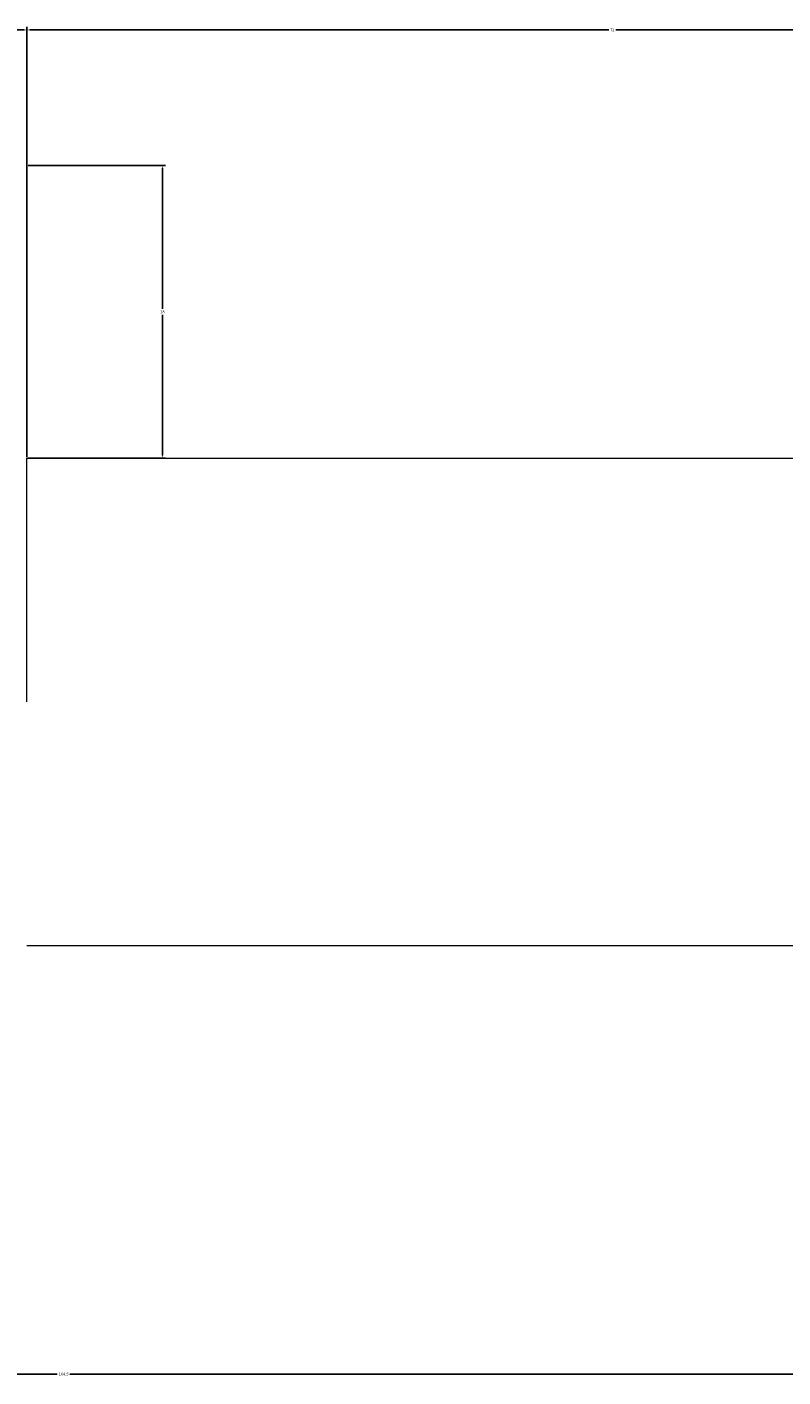
# Model space of a CAD drawing. Units: millimetres. Extents: x 2117 to 2298, y 1328 to 1411.
# Tile 2 of 3: x 2205 to 2252, y 1328 to 1411. Entities that reach past the tile are written whole.
import ezdxf

# ---------------------------------------------------------------- set-up
doc = ezdxf.new("R2010")
doc.units = ezdxf.units.MM
doc.layers.add('M-CONS', color=8, linetype='Continuous', lineweight=18)
doc.layers.add('M-DIMS', color=2, linetype='Continuous', lineweight=18)
doc.styles.get("Standard").update_dxf_attribs({"font": 'arial.ttf'})
doc.dimstyles.get("Standard").update_dxf_attribs({"dimtxt": 0.18, "dimasz": 0.18, "dimexe": 0.18, "dimexo": 0.0625, "dimgap": 0.09, "dimtad": 0, "dimtih": 1, "dimtoh": 1, "dimdec": 4, "dimzin": 0, "dimdsep": 46, "dimtxsty": 'Standard', "dimcen": 0.09, "dimadec": 0, "dimazin": 0, "dimtfac": 1, "dimtdec": 4, "dimtofl": 0, "dimtmove": 0, "dimatfit": 3, "dimfxl": 1, "dimtolj": 1, "dimtzin": 0, "dimarcsym": 0})

# ---------------------------------------------------------------- blocks, each defined once
blk = doc.blocks.new('*D6')
at = {"layer": 'Defpoints', "color": 0, "transparency": 16777216}
for p in [(2205.416, 1411.113), (2187.416, 1402.783), (2205.416, 1402.783)]:
    blk.add_point(p, dxfattribs=at)
at = {"layer": 'M-DIMS', "color": 0, "lineweight": -2, "transparency": 16777216}
for p, q in [((2187.416, 1402.845), (2187.416, 1411.293)), ((2187.596, 1411.113), (2196.205, 1411.113)), ((2205.236, 1411.113), (2196.627, 1411.113)), ((2205.416, 1402.845), (2205.416, 1411.293))]:
    blk.add_line(p, q, dxfattribs=at)
at = {"layer": 'M-DIMS', "color": 0, "transparency": 16777216}
for points in [[(2187.596, 1411.143), (2187.596, 1411.083), (2187.416, 1411.113)], [(2205.236, 1411.143), (2205.236, 1411.083), (2205.416, 1411.113)]]:
    blk.add_solid(points, dxfattribs=at)
at = {"layer": 'M-DIMS', "color": 0, "transparency": 16777216, "insert": (2196.416, 1411.113), "char_height": 0.18, "attachment_point": 5}
blk.add_mtext('\\A1;18', dxfattribs=at)
blk = doc.blocks.new('*D7')
at = {"layer": 'Defpoints', "color": 0, "transparency": 16777216}
for p in [(2277.416, 1411.113), (2205.416, 1384.783), (2277.416, 1384.783)]:
    blk.add_point(p, dxfattribs=at)
at = {"layer": 'M-DIMS', "color": 0, "lineweight": -2, "transparency": 16777216}
for p, q in [((2205.416, 1384.845), (2205.416, 1411.293)), ((2205.596, 1411.113), (2241.199, 1411.113)), ((2277.236, 1411.113), (2241.633, 1411.113)), ((2277.416, 1384.845), (2277.416, 1411.293))]:
    blk.add_line(p, q, dxfattribs=at)
at = {"layer": 'M-DIMS', "color": 0, "transparency": 16777216}
for points in [[(2205.596, 1411.143), (2205.596, 1411.083), (2205.416, 1411.113)], [(2277.236, 1411.143), (2277.236, 1411.083), (2277.416, 1411.113)]]:
    blk.add_solid(points, dxfattribs=at)
at = {"layer": 'M-DIMS', "color": 0, "transparency": 16777216, "insert": (2241.416, 1411.113), "char_height": 0.18, "attachment_point": 5}
blk.add_mtext('\\A1;72', dxfattribs=at)
blk = doc.blocks.new('*D9')
at = {"layer": 'Defpoints', "color": 0, "transparency": 16777216}
for p in [(2205.416, 1402.783), (2205.416, 1384.783), (2213.746, 1384.783)]:
    blk.add_point(p, dxfattribs=at)
at = {"layer": 'M-DIMS', "color": 0, "lineweight": -2, "transparency": 16777216}
for p, q in [((2205.479, 1402.783), (2213.926, 1402.783)), ((2213.746, 1402.603), (2213.746, 1393.965)), ((2213.746, 1384.963), (2213.746, 1393.601)), ((2205.479, 1384.783), (2213.926, 1384.783))]:
    blk.add_line(p, q, dxfattribs=at)
at = {"layer": 'M-DIMS', "color": 0, "transparency": 16777216}
for points in [[(2213.716, 1402.603), (2213.776, 1402.603), (2213.746, 1402.783)], [(2213.716, 1384.963), (2213.776, 1384.963), (2213.746, 1384.783)]]:
    blk.add_solid(points, dxfattribs=at)
at = {"layer": 'M-DIMS', "color": 0, "transparency": 16777216, "insert": (2213.746, 1393.783), "char_height": 0.18, "attachment_point": 5}
blk.add_mtext('\\A1;18', dxfattribs=at)
blk = doc.blocks.new('*D12')
at = {"layer": 'Defpoints', "color": 0, "transparency": 16777216}
for p in [(2125.416, 1369.783), (2289.916, 1354.783), (2289.916, 1328.453)]:
    blk.add_point(p, dxfattribs=at)
at = {"layer": 'M-DIMS', "color": 0, "lineweight": -2, "transparency": 16777216}
for p, q in [((2125.416, 1369.72), (2125.416, 1328.273)), ((2289.916, 1354.72), (2289.916, 1328.273)), ((2125.596, 1328.453), (2207.28, 1328.453)), ((2289.736, 1328.453), (2208.052, 1328.453))]:
    blk.add_line(p, q, dxfattribs=at)
at = {"layer": 'M-DIMS', "color": 0, "transparency": 16777216}
for points in [[(2125.596, 1328.483), (2125.596, 1328.423), (2125.416, 1328.453)], [(2289.736, 1328.483), (2289.736, 1328.423), (2289.916, 1328.453)]]:
    blk.add_solid(points, dxfattribs=at)
at = {"layer": 'M-DIMS', "color": 0, "transparency": 16777216, "insert": (2207.666, 1328.453), "char_height": 0.18, "attachment_point": 5}
blk.add_mtext('\\A1;164.5', dxfattribs=at)

msp = doc.modelspace()

# ---------------------------------------------------------------- linework, layer by layer
at = {"layer": 'M-CONS'}
msp.add_lwpolyline([(2205.416, 1369.783), (2205.416, 1384.783), (2277.416, 1384.783), (2277.416, 1354.783), (2205.416, 1354.783)], dxfattribs=at)

# ---------------------------------------------------------------- dimensions: what is measured, and where the dimension line sits
at = {"layer": 'M-DIMS'}
for base, p1, p2, override, picture, middle in [((2205.416, 1411.113), (2187.416, 1402.783), (2205.416, 1402.783), {"dimdec": 0, "dimlfac": 1, "dimrnd": 0, "dimzin": 0, "dimdsep": 46, "dimlunit": 2}, '*D6', (2196.416, 1411.113)), ((2277.416, 1411.113), (2205.416, 1384.783), (2277.416, 1384.783), {"dimdec": 0, "dimlfac": 1, "dimrnd": 0, "dimzin": 0, "dimdsep": 46, "dimlunit": 2}, '*D7', (2241.416, 1411.113)), ((2289.916, 1328.453), (2125.416, 1369.783), (2289.916, 1354.783), {"dimdec": 1, "dimlfac": 1, "dimrnd": 0, "dimzin": 0, "dimdsep": 46, "dimlunit": 2}, '*D12', (2207.666, 1328.453))]:
    dim = msp.add_linear_dim(base=base, p1=p1, p2=p2, dimstyle='Standard', override=override, dxfattribs=at)
    dim.commit()
    dim.dimension.update_dxf_attribs({"geometry": picture, "text_midpoint": middle})
dim = msp.add_linear_dim(base=(2213.746, 1384.783), p1=(2205.416, 1402.783), p2=(2205.416, 1384.783), angle=270, dimstyle='Standard', override={"dimdec": 0, "dimlfac": 1, "dimrnd": 0, "dimzin": 0, "dimdsep": 46, "dimlunit": 2}, dxfattribs=at)
dim.commit()
dim.dimension.update_dxf_attribs({"geometry": '*D9', "text_midpoint": (2213.746, 1393.783)})

doc.saveas('drawing.dxf')
